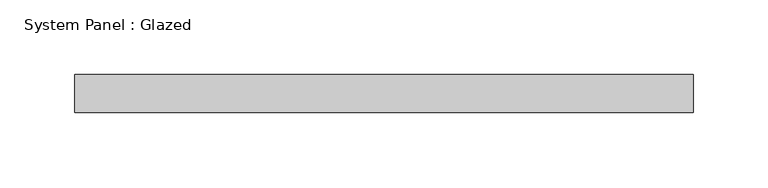
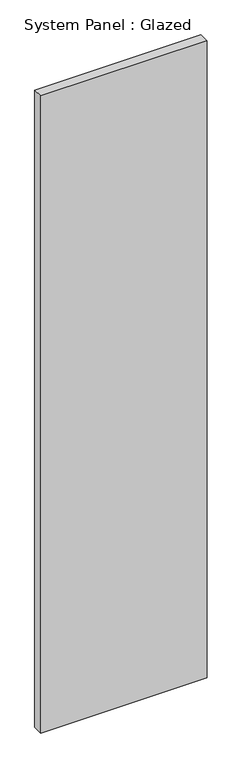
"""IFC4 building model written with IfcOpenShell, lengths in millimetres: plate geometry, System Panel : Glazed."""

from ifc_helpers import new_model, si_unit, origin, origin_with_axes, place, context, project, spatial, polyline, outline, extrude, source, transform, mapped, element, save


def system_panel_glazed_42f26034(model_context):
    return source(origin(), model_context, "Body", "SweptSolid", [
        extrude(outline(polyline([(206.375, 19.05), (-206.375, 19.05), (-206.375, 44.45), (206.375, 44.45), (206.375, 19.05)])), origin_with_axes(), (0.0, 0.0, 1.0), 1669.4671151),
    ])


if __name__ == "__main__":
    model = new_model("IFC4")
    model_context = context("Model", 3, world=origin())
    ifc_project = project(units=[si_unit("LENGTHUNIT", "METRE", prefix="MILLI")], contexts=[model_context])
    site = spatial("IfcSite", under=ifc_project)
    building = spatial("IfcBuilding", under=site)
    placement = place(None, origin())
    system_panel_glazed_shape = system_panel_glazed_42f26034(model_context)
    element("IfcPlate", 1, ObjectType="System Panel : Glazed", at=placement, inside=building, context=model_context, shape_type="MappedRepresentation", body=[
        mapped(system_panel_glazed_shape, transform((0.0, 0.0, 0.0), x_axis=(1.0, 0.0, 0.0), y_axis=(0.0, 1.0, 0.0), z_axis=(0.0, 0.0, 1.0))),
    ])
    save(model, "model.ifc")

# Revit data of these elements
# Type "System Panel : Glazed"
#   Construction Type Id = "GSP4R"
#   Analytic Construction = "1/8 in Pilkington single glazing"
#   Visual Light Transmittance = 0.9
#   Solar Heat Gain Coefficient = 0.86
#   Heat Transfer Coefficient (U) = 1.18115 BTU/(h·ft²·°F)
#   Define Thermal Properties by = 1
# Element 1 (IfcPlate, "System Panel : Glazed")
#   Materials on its faces: "Glass"
# Materials
#   "Glass": class "Glass", colour RGB 0 128 192, transparency 0.75, Description = "Soda Lime Glass", Cost = 0
